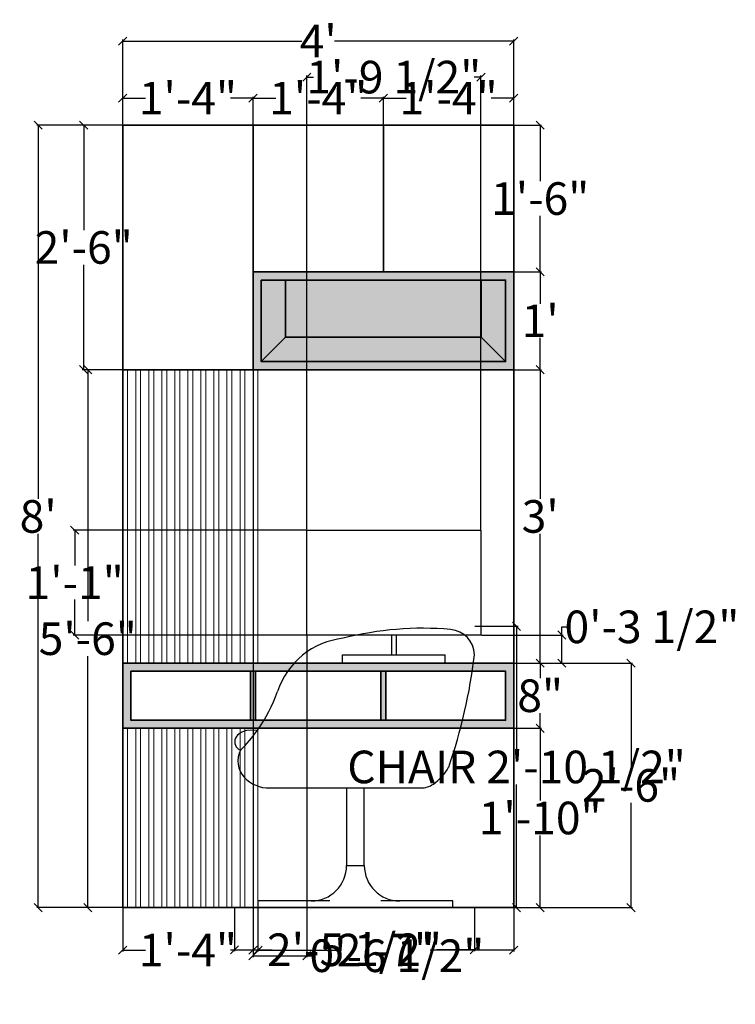
# Model space of a CAD drawing. Units: inches. Extents: x 1 to 89, y 9 to 130.
import ezdxf

# ---------------------------------------------------------------- set-up
doc = ezdxf.new("R2010")
doc.units = ezdxf.units.IN
doc.header["$MEASUREMENT"] = 0
for name, color, linetype, lineweight in [('A-ANNO-DIMS', 2, 'Continuous', 18), ('A-ELEV', 7, 'Continuous', 35), ('A-ELEV-PATT', 8, 'Continuous', 13), ('A-FURN', 8, 'Continuous', 25)]:
    doc.layers.add(name, color=color, linetype=linetype, lineweight=lineweight)
doc.styles.get("Standard").update_dxf_attribs({"font": 'arial.ttf'})
doc.dimstyles.get("Standard").update_dxf_attribs({"dimtxt": 4, "dimasz": 1, "dimexe": 0.18, "dimexo": 0.0625, "dimgap": 0.09, "dimtad": 0, "dimtih": 1, "dimtoh": 1, "dimdec": 0, "dimzin": 0, "dimdsep": 46, "dimlunit": 4, "dimtxsty": 'Standard', "dimblk": 'OBLIQUE', "dimcen": 0.09, "dimadec": 0, "dimazin": 0, "dimtfac": 1, "dimtdec": 0, "dimtofl": 0, "dimtmove": 0, "dimatfit": 3, "dimldrblk": 'OBLIQUE', "dimfxl": 1, "dimtolj": 1, "dimtzin": 0, "dimarcsym": 0})

# ---------------------------------------------------------------- blocks, each defined once
blk = doc.blocks.new('A$C2F5F5597')
at = {"ltscale": 20}
for p, q in [((51.1, 400), (27.4, 399.3)), ((79, 270), (252.2, 270)), ((252.2, 270), (252.2, 95)), ((292.2, 95), (292.2, 270)), ((292.2, 270), (419.9, 270)), ((252.2, 95), (292.2, 95)), ((172.2, 15), (52.2, 15)), ((52.2, 15), (52.2, 0)), ((214.7, 15), (52.2, 15)), ((52.2, 0), (492.2, 0)), ((492.2, 15), (329.7, 15)), ((492.2, 15), (372.2, 15)), ((492.2, 0), (492.2, 15))]:
    blk.add_line(p, q, dxfattribs=at)
blk.add_line((252.2, 270), (292.2, 270))
for centre, radius, start, end in [((424, -95.9), 726, 85.0159, 104.3072), ((482.6, 569.3), 58.2, 1.2474, 85.5637), ((264.6, 431.4), 177.3, 96.4526, 161.6024), ((-670.9, 714.7), 1220.3, 340.9618, 353.2158), ((-231.8, 601.9), 347.5, 324.4887, 340.7516), ((-231.8, 601.9), 347.5, 314.7292, 324.4887), ((20.7, 374.3), 20.9, 157.0939, 247.6023), ((31.5, 364.8), 34.8, 96.6901, 149.4967), ((60.1, 330.5), 53.3, 152.6544, 222.8556), ((385.8, 370), 110.5, 304.2659, 331.155), ((77, 346.6), 76.7, 223.0738, 271.4724), ((419.9, 320), 50, 270, 304.2659), ((172.2, 95), 80, 270, 0), ((372.2, 95), 80, 180, 270)]:
    blk.add_arc(centre, radius, start, end, dxfattribs=at)
blk = doc.blocks.new('_Oblique')
at = {"color": 0, "linetype": 'ByBlock', "lineweight": -2}
blk.add_line((-0.5, -0.5), (0.5, 0.5), dxfattribs=at)
blk = doc.blocks.new('*D3')
at = {"layer": 'A-ANNO-DIMS', "color": 0, "lineweight": -2, "transparency": 16777216}
for p, q in [((13.37, 116.69), (13.37, 127.12)), ((13.37, 126.94), (35.36, 126.94)), ((61.37, 126.94), (39.38, 126.94)), ((61.37, 116.69), (61.37, 127.12))]:
    blk.add_line(p, q, dxfattribs=at)
at = {"layer": 'Defpoints', "color": 0, "transparency": 16777216}
for p in [(61.37, 126.94), (13.37, 116.62), (61.37, 116.62)]:
    blk.add_point(p, dxfattribs=at)
at = {"layer": 'A-ANNO-DIMS', "color": 0, "lineweight": -2, "transparency": 16777216, "rotation": 180}
blk.add_blockref('_Oblique', (13.37, 126.94), dxfattribs=at)
at = {"layer": 'A-ANNO-DIMS', "color": 0, "lineweight": -2, "transparency": 16777216}
blk.add_blockref('_Oblique', (61.37, 126.94), dxfattribs=at)
at = {"layer": 'A-ANNO-DIMS', "color": 0, "transparency": 16777216, "insert": (37.37, 126.94), "char_height": 4, "attachment_point": 5}
blk.add_mtext("\\A1;4'", dxfattribs=at)
blk = doc.blocks.new('*D4')
at = {"layer": 'A-ANNO-DIMS', "color": 0, "lineweight": -2, "transparency": 16777216}
for p, q in [((13.37, 116.69), (13.37, 120.12)), ((13.37, 119.94), (16.15, 119.94)), ((29.37, 119.94), (26.59, 119.94)), ((29.37, 116.69), (29.37, 120.12))]:
    blk.add_line(p, q, dxfattribs=at)
at = {"layer": 'Defpoints', "color": 0, "transparency": 16777216}
for p in [(29.37, 119.94), (13.37, 116.62), (29.37, 116.62)]:
    blk.add_point(p, dxfattribs=at)
at = {"layer": 'A-ANNO-DIMS', "color": 0, "lineweight": -2, "transparency": 16777216, "rotation": 180}
blk.add_blockref('_Oblique', (13.37, 119.94), dxfattribs=at)
at = {"layer": 'A-ANNO-DIMS', "color": 0, "lineweight": -2, "transparency": 16777216}
blk.add_blockref('_Oblique', (29.37, 119.94), dxfattribs=at)
at = {"layer": 'A-ANNO-DIMS', "color": 0, "transparency": 16777216, "insert": (21.37, 119.94), "char_height": 4, "attachment_point": 5}
blk.add_mtext('\\A1;1\'-4"', dxfattribs=at)
blk = doc.blocks.new('*D5')
at = {"layer": 'A-ANNO-DIMS', "color": 0, "lineweight": -2, "transparency": 16777216}
for p, q in [((29.37, 116.69), (29.37, 120.12)), ((29.37, 119.94), (32.15, 119.94)), ((45.37, 119.94), (42.59, 119.94)), ((45.37, 116.69), (45.37, 120.12))]:
    blk.add_line(p, q, dxfattribs=at)
at = {"layer": 'Defpoints', "color": 0, "transparency": 16777216}
for p in [(45.37, 119.94), (29.37, 116.62), (45.37, 116.62)]:
    blk.add_point(p, dxfattribs=at)
at = {"layer": 'A-ANNO-DIMS', "color": 0, "lineweight": -2, "transparency": 16777216, "rotation": 180}
blk.add_blockref('_Oblique', (29.37, 119.94), dxfattribs=at)
at = {"layer": 'A-ANNO-DIMS', "color": 0, "lineweight": -2, "transparency": 16777216}
blk.add_blockref('_Oblique', (45.37, 119.94), dxfattribs=at)
at = {"layer": 'A-ANNO-DIMS', "color": 0, "transparency": 16777216, "insert": (37.37, 119.94), "char_height": 4, "attachment_point": 5}
blk.add_mtext('\\A1;1\'-4"', dxfattribs=at)
blk = doc.blocks.new('*D6')
at = {"layer": 'A-ANNO-DIMS', "color": 0, "lineweight": -2, "transparency": 16777216}
for p, q in [((45.37, 116.69), (45.37, 120.12)), ((45.37, 119.94), (48.15, 119.94)), ((61.37, 119.94), (58.59, 119.94)), ((61.37, 116.69), (61.37, 120.12))]:
    blk.add_line(p, q, dxfattribs=at)
at = {"layer": 'Defpoints', "color": 0, "transparency": 16777216}
for p in [(61.37, 119.94), (45.37, 116.62), (61.37, 116.62)]:
    blk.add_point(p, dxfattribs=at)
at = {"layer": 'A-ANNO-DIMS', "color": 0, "lineweight": -2, "transparency": 16777216, "rotation": 180}
blk.add_blockref('_Oblique', (45.37, 119.94), dxfattribs=at)
at = {"layer": 'A-ANNO-DIMS', "color": 0, "lineweight": -2, "transparency": 16777216}
blk.add_blockref('_Oblique', (61.37, 119.94), dxfattribs=at)
at = {"layer": 'A-ANNO-DIMS', "color": 0, "transparency": 16777216, "insert": (53.37, 119.94), "char_height": 4, "attachment_point": 5}
blk.add_mtext('\\A1;1\'-4"', dxfattribs=at)
blk = doc.blocks.new('*D7')
at = {"layer": 'A-ANNO-DIMS', "color": 0, "lineweight": -2, "transparency": 16777216}
for p, q in [((61.43, 116.62), (64.8, 116.62)), ((64.62, 116.62), (64.62, 109.76)), ((64.62, 98.62), (64.62, 105.49)), ((61.43, 98.62), (64.8, 98.62))]:
    blk.add_line(p, q, dxfattribs=at)
at = {"layer": 'Defpoints', "color": 0, "transparency": 16777216}
for p in [(61.37, 116.62), (61.37, 98.62), (64.62, 98.62)]:
    blk.add_point(p, dxfattribs=at)
at = {"layer": 'A-ANNO-DIMS', "color": 0, "lineweight": -2, "transparency": 16777216}
for p, rotation in [((64.62, 116.62), 90), ((64.62, 98.62), 270)]:
    blk.add_blockref('_Oblique', p, dxfattribs=dict(at, rotation=rotation))
at = {"layer": 'A-ANNO-DIMS', "color": 0, "transparency": 16777216, "insert": (64.62, 107.62), "char_height": 4, "attachment_point": 5}
blk.add_mtext('\\A1;1\'-6"', dxfattribs=at)
blk = doc.blocks.new('*D8')
at = {"layer": 'A-ANNO-DIMS', "color": 0, "lineweight": -2, "transparency": 16777216}
for p, q in [((61.43, 98.62), (64.8, 98.62)), ((64.62, 98.62), (64.62, 94.72)), ((64.62, 86.62), (64.62, 90.53)), ((61.43, 86.62), (64.8, 86.62))]:
    blk.add_line(p, q, dxfattribs=at)
at = {"layer": 'Defpoints', "color": 0, "transparency": 16777216}
for p in [(61.37, 98.62), (64.62, 98.62), (61.37, 86.62)]:
    blk.add_point(p, dxfattribs=at)
at = {"layer": 'A-ANNO-DIMS', "color": 0, "lineweight": -2, "transparency": 16777216}
for p, rotation in [((64.62, 98.62), 90), ((64.62, 86.62), 270)]:
    blk.add_blockref('_Oblique', p, dxfattribs=dict(at, rotation=rotation))
at = {"layer": 'A-ANNO-DIMS', "color": 0, "transparency": 16777216, "insert": (64.62, 92.62), "char_height": 4, "attachment_point": 5}
blk.add_mtext("\\A1;1'", dxfattribs=at)
blk = doc.blocks.new('*D9')
at = {"layer": 'A-ANNO-DIMS', "color": 0, "lineweight": -2, "transparency": 16777216}
for p, q in [((61.43, 86.62), (64.8, 86.62)), ((64.62, 86.62), (64.62, 70.76)), ((64.62, 50.62), (64.62, 66.49)), ((61.43, 50.62), (64.8, 50.62))]:
    blk.add_line(p, q, dxfattribs=at)
at = {"layer": 'Defpoints', "color": 0, "transparency": 16777216}
for p in [(61.37, 86.62), (61.37, 50.62), (64.62, 50.62)]:
    blk.add_point(p, dxfattribs=at)
at = {"layer": 'A-ANNO-DIMS', "color": 0, "lineweight": -2, "transparency": 16777216}
for p, rotation in [((64.62, 86.62), 90), ((64.62, 50.62), 270)]:
    blk.add_blockref('_Oblique', p, dxfattribs=dict(at, rotation=rotation))
at = {"layer": 'A-ANNO-DIMS', "color": 0, "transparency": 16777216, "insert": (64.62, 68.62), "char_height": 4, "attachment_point": 5}
blk.add_mtext("\\A1;3'", dxfattribs=at)
blk = doc.blocks.new('*D10')
at = {"layer": 'A-ANNO-DIMS', "color": 0, "lineweight": -2, "transparency": 16777216}
for p, q in [((61.43, 50.62), (64.8, 50.62)), ((64.62, 50.62), (64.62, 48.76)), ((64.62, 42.62), (64.62, 44.49)), ((61.43, 42.62), (64.8, 42.62))]:
    blk.add_line(p, q, dxfattribs=at)
at = {"layer": 'Defpoints', "color": 0, "transparency": 16777216}
for p in [(61.37, 50.62), (61.37, 42.62), (64.62, 42.62)]:
    blk.add_point(p, dxfattribs=at)
at = {"layer": 'A-ANNO-DIMS', "color": 0, "lineweight": -2, "transparency": 16777216}
for p, rotation in [((64.62, 50.62), 90), ((64.62, 42.62), 270)]:
    blk.add_blockref('_Oblique', p, dxfattribs=dict(at, rotation=rotation))
at = {"layer": 'A-ANNO-DIMS', "color": 0, "transparency": 16777216, "insert": (64.62, 46.62), "char_height": 4, "attachment_point": 5}
blk.add_mtext('\\A1;8"', dxfattribs=at)
blk = doc.blocks.new('*D11')
at = {"layer": 'A-ANNO-DIMS', "color": 0, "lineweight": -2, "transparency": 16777216}
for p, q in [((61.43, 42.62), (64.8, 42.62)), ((64.62, 42.62), (64.62, 33.76)), ((64.62, 20.62), (64.62, 29.49)), ((61.43, 20.62), (64.8, 20.62))]:
    blk.add_line(p, q, dxfattribs=at)
at = {"layer": 'Defpoints', "color": 0, "transparency": 16777216}
for p in [(61.37, 42.62), (61.37, 20.62), (64.62, 20.62)]:
    blk.add_point(p, dxfattribs=at)
at = {"layer": 'A-ANNO-DIMS', "color": 0, "lineweight": -2, "transparency": 16777216}
for p, rotation in [((64.62, 42.62), 90), ((64.62, 20.62), 270)]:
    blk.add_blockref('_Oblique', p, dxfattribs=dict(at, rotation=rotation))
at = {"layer": 'A-ANNO-DIMS', "color": 0, "transparency": 16777216, "insert": (64.62, 31.62), "char_height": 4, "attachment_point": 5}
blk.add_mtext('\\A1;1\'-10"', dxfattribs=at)
blk = doc.blocks.new('*D12')
at = {"layer": 'A-ANNO-DIMS', "color": 0, "lineweight": -2, "transparency": 16777216}
for p, q in [((61.43, 50.62), (75.95, 50.62)), ((75.77, 50.62), (75.77, 37.76)), ((75.77, 20.62), (75.77, 33.49)), ((61.43, 20.62), (75.95, 20.62))]:
    blk.add_line(p, q, dxfattribs=at)
at = {"layer": 'Defpoints', "color": 0, "transparency": 16777216}
for p in [(61.37, 50.62), (61.37, 20.62), (75.77, 20.62)]:
    blk.add_point(p, dxfattribs=at)
at = {"layer": 'A-ANNO-DIMS', "color": 0, "lineweight": -2, "transparency": 16777216}
for p, rotation in [((75.77, 50.62), 90), ((75.77, 20.62), 270)]:
    blk.add_blockref('_Oblique', p, dxfattribs=dict(at, rotation=rotation))
at = {"layer": 'A-ANNO-DIMS', "color": 0, "transparency": 16777216, "insert": (75.77, 35.62), "char_height": 4, "attachment_point": 5}
blk.add_mtext('\\A1;2\'-6"', dxfattribs=at)
blk = doc.blocks.new('*D13')
at = {"layer": 'A-ANNO-DIMS', "color": 0, "lineweight": -2, "transparency": 16777216}
for p, q in [((29.37, 86.56), (29.37, 15.23)), ((13.37, 20.56), (13.37, 15.23)), ((13.37, 15.41), (16.15, 15.41)), ((29.37, 15.41), (26.59, 15.41))]:
    blk.add_line(p, q, dxfattribs=at)
at = {"layer": 'Defpoints', "color": 0, "transparency": 16777216}
for p in [(29.37, 86.62), (13.37, 20.62), (29.37, 15.41)]:
    blk.add_point(p, dxfattribs=at)
at = {"layer": 'A-ANNO-DIMS', "color": 0, "lineweight": -2, "transparency": 16777216, "rotation": 180}
blk.add_blockref('_Oblique', (13.37, 15.41), dxfattribs=at)
at = {"layer": 'A-ANNO-DIMS', "color": 0, "lineweight": -2, "transparency": 16777216}
blk.add_blockref('_Oblique', (29.37, 15.41), dxfattribs=at)
at = {"layer": 'A-ANNO-DIMS', "color": 0, "transparency": 16777216, "insert": (21.37, 15.41), "char_height": 4, "attachment_point": 5}
blk.add_mtext('\\A1;1\'-4"', dxfattribs=at)
blk = doc.blocks.new('*D14')
at = {"layer": 'A-ANNO-DIMS', "color": 0, "lineweight": -2, "transparency": 16777216}
for p, q in [((61.37, 86.56), (61.37, 15.23)), ((29.97, 20.56), (29.97, 15.23)), ((29.97, 15.41), (40.23, 15.41)), ((61.37, 15.41), (51.11, 15.41))]:
    blk.add_line(p, q, dxfattribs=at)
at = {"layer": 'Defpoints', "color": 0, "transparency": 16777216}
for p in [(61.37, 86.62), (29.97, 20.62), (61.37, 15.41)]:
    blk.add_point(p, dxfattribs=at)
at = {"layer": 'A-ANNO-DIMS', "color": 0, "lineweight": -2, "transparency": 16777216, "rotation": 180}
blk.add_blockref('_Oblique', (29.97, 15.41), dxfattribs=at)
at = {"layer": 'A-ANNO-DIMS', "color": 0, "lineweight": -2, "transparency": 16777216}
blk.add_blockref('_Oblique', (61.37, 15.41), dxfattribs=at)
at = {"layer": 'A-ANNO-DIMS', "color": 0, "transparency": 16777216, "insert": (45.67, 15.41), "char_height": 4, "attachment_point": 5}
blk.add_mtext('\\A1;2\'-7"', dxfattribs=at)
blk = doc.blocks.new('*D15')
at = {"layer": 'A-ANNO-DIMS', "color": 0, "lineweight": -2, "transparency": 16777216}
for p, q in [((13.31, 86.62), (8.9, 86.62)), ((9.08, 86.62), (9.08, 55.76)), ((9.08, 20.62), (9.08, 51.49)), ((13.31, 20.62), (8.9, 20.62))]:
    blk.add_line(p, q, dxfattribs=at)
at = {"layer": 'Defpoints', "color": 0, "transparency": 16777216}
for p in [(13.37, 86.62), (9.08, 20.62), (13.37, 20.62)]:
    blk.add_point(p, dxfattribs=at)
at = {"layer": 'A-ANNO-DIMS', "color": 0, "lineweight": -2, "transparency": 16777216}
for p, rotation in [((9.08, 86.62), 90), ((9.08, 20.62), 270)]:
    blk.add_blockref('_Oblique', p, dxfattribs=dict(at, rotation=rotation))
at = {"layer": 'A-ANNO-DIMS', "color": 0, "transparency": 16777216, "insert": (9.08, 53.62), "char_height": 4, "attachment_point": 5}
blk.add_mtext('\\A1;5\'-6"', dxfattribs=at)
blk = doc.blocks.new('*D16')
at = {"layer": 'A-ANNO-DIMS', "color": 0, "lineweight": -2, "transparency": 16777216}
for p, q in [((13.31, 116.62), (8.4, 116.62)), ((8.58, 116.62), (8.58, 103.76)), ((8.58, 86.62), (8.58, 99.49)), ((13.31, 86.62), (8.4, 86.62))]:
    blk.add_line(p, q, dxfattribs=at)
at = {"layer": 'Defpoints', "color": 0, "transparency": 16777216}
for p in [(13.37, 116.62), (8.58, 86.62), (13.37, 86.62)]:
    blk.add_point(p, dxfattribs=at)
at = {"layer": 'A-ANNO-DIMS', "color": 0, "lineweight": -2, "transparency": 16777216}
for p, rotation in [((8.58, 116.62), 90), ((8.58, 86.62), 270)]:
    blk.add_blockref('_Oblique', p, dxfattribs=dict(at, rotation=rotation))
at = {"layer": 'A-ANNO-DIMS', "color": 0, "transparency": 16777216, "insert": (8.58, 101.62), "char_height": 4, "attachment_point": 5}
blk.add_mtext('\\A1;2\'-6"', dxfattribs=at)
blk = doc.blocks.new('*D17')
at = {"layer": 'A-ANNO-DIMS', "color": 0, "lineweight": -2, "transparency": 16777216}
for p, q in [((13.31, 116.62), (2.81, 116.62)), ((2.99, 116.62), (2.99, 70.76)), ((2.99, 20.62), (2.99, 66.49)), ((13.91, 20.62), (2.81, 20.62))]:
    blk.add_line(p, q, dxfattribs=at)
at = {"layer": 'Defpoints', "color": 0, "transparency": 16777216}
for p in [(13.37, 116.62), (2.99, 20.62), (13.97, 20.62)]:
    blk.add_point(p, dxfattribs=at)
at = {"layer": 'A-ANNO-DIMS', "color": 0, "lineweight": -2, "transparency": 16777216}
for p, rotation in [((2.99, 116.62), 90), ((2.99, 20.62), 270)]:
    blk.add_blockref('_Oblique', p, dxfattribs=dict(at, rotation=rotation))
at = {"layer": 'A-ANNO-DIMS', "color": 0, "transparency": 16777216, "insert": (2.99, 68.62), "char_height": 4, "attachment_point": 5}
blk.add_mtext("\\A1;8'", dxfattribs=at)
blk = doc.blocks.new('*D18')
at = {"layer": 'A-ANNO-DIMS', "color": 0, "lineweight": -2, "transparency": 16777216}
for p, q in [((56.61, 55.14), (61.9, 55.14)), ((61.72, 55.14), (61.72, 40.04)), ((61.72, 20.62), (61.72, 35.72)), ((56.61, 20.62), (61.9, 20.62))]:
    blk.add_line(p, q, dxfattribs=at)
at = {"layer": 'Defpoints', "color": 0, "transparency": 16777216}
for p in [(56.54, 55.14), (61.72, 55.14), (56.54, 20.62)]:
    blk.add_point(p, dxfattribs=at)
at = {"layer": 'A-ANNO-DIMS', "color": 0, "lineweight": -2, "transparency": 16777216}
for p, rotation in [((61.72, 55.14), 90), ((61.72, 20.62), 270)]:
    blk.add_blockref('_Oblique', p, dxfattribs=dict(at, rotation=rotation))
at = {"layer": 'A-ANNO-DIMS', "color": 0, "transparency": 16777216, "insert": (61.72, 37.88), "char_height": 4, "attachment_point": 5}
blk.add_mtext('\\A1;CHAIR 2\'-10 1/2"', dxfattribs=at)
blk = doc.blocks.new('*D19')
at = {"layer": 'A-ANNO-DIMS', "color": 0, "lineweight": -2, "transparency": 16777216}
for p, q in [((27.09, 20.56), (27.09, 15.27)), ((56.54, 20.56), (56.54, 15.27)), ((27.09, 15.45), (31.72, 15.45)), ((56.54, 15.45), (51.92, 15.45))]:
    blk.add_line(p, q, dxfattribs=at)
at = {"layer": 'Defpoints', "color": 0, "transparency": 16777216}
for p in [(27.09, 20.62), (56.54, 20.62), (56.54, 15.45)]:
    blk.add_point(p, dxfattribs=at)
at = {"layer": 'A-ANNO-DIMS', "color": 0, "lineweight": -2, "transparency": 16777216, "rotation": 180}
blk.add_blockref('_Oblique', (27.09, 15.45), dxfattribs=at)
at = {"layer": 'A-ANNO-DIMS', "color": 0, "lineweight": -2, "transparency": 16777216}
blk.add_blockref('_Oblique', (56.54, 15.45), dxfattribs=at)
at = {"layer": 'A-ANNO-DIMS', "color": 0, "transparency": 16777216, "insert": (41.82, 15.45), "char_height": 4, "attachment_point": 5}
blk.add_mtext('\\A1;2\'-5 1/2"', dxfattribs=at)
blk = doc.blocks.new('*D20')
at = {"layer": 'A-ANNO-DIMS', "color": 0, "lineweight": -2, "transparency": 16777216}
for p, q in [((35.96, 67), (35.96, 122.7)), ((35.96, 122.52), (36.78, 122.52)), ((57.35, 122.52), (56.53, 122.52)), ((57.35, 67), (57.35, 122.7))]:
    blk.add_line(p, q, dxfattribs=at)
at = {"layer": 'Defpoints', "color": 0, "transparency": 16777216}
for p in [(57.35, 122.52), (35.96, 66.93), (57.35, 66.93)]:
    blk.add_point(p, dxfattribs=at)
at = {"layer": 'A-ANNO-DIMS', "color": 0, "lineweight": -2, "transparency": 16777216, "rotation": 180}
blk.add_blockref('_Oblique', (35.96, 122.52), dxfattribs=at)
at = {"layer": 'A-ANNO-DIMS', "color": 0, "lineweight": -2, "transparency": 16777216}
blk.add_blockref('_Oblique', (57.35, 122.52), dxfattribs=at)
at = {"layer": 'A-ANNO-DIMS', "color": 0, "transparency": 16777216, "insert": (46.65, 122.52), "char_height": 4, "attachment_point": 5}
blk.add_mtext('\\A1;1\'-9 1/2"', dxfattribs=at)
blk = doc.blocks.new('*D21')
at = {"layer": 'A-ANNO-DIMS', "color": 0, "lineweight": -2, "transparency": 16777216}
for p, q in [((35.9, 66.93), (7.29, 66.93)), ((7.47, 66.93), (7.47, 62.6)), ((7.47, 54.07), (7.47, 58.41)), ((35.9, 54.07), (7.29, 54.07))]:
    blk.add_line(p, q, dxfattribs=at)
at = {"layer": 'Defpoints', "color": 0, "transparency": 16777216}
for p in [(7.47, 66.93), (35.96, 66.93), (35.96, 54.07)]:
    blk.add_point(p, dxfattribs=at)
at = {"layer": 'A-ANNO-DIMS', "color": 0, "lineweight": -2, "transparency": 16777216}
for p, rotation in [((7.47, 66.93), 90), ((7.47, 54.07), 270)]:
    blk.add_blockref('_Oblique', p, dxfattribs=dict(at, rotation=rotation))
at = {"layer": 'A-ANNO-DIMS', "color": 0, "transparency": 16777216, "insert": (7.47, 60.5), "char_height": 4, "attachment_point": 5}
blk.add_mtext('\\A1;1\'-1"', dxfattribs=at)
blk = doc.blocks.new('*D22')
at = {"layer": 'A-ANNO-DIMS', "color": 0, "lineweight": -2, "transparency": 16777216}
for p, q in [((67.27, 54.07), (67.27, 55.07)), ((67.27, 55.07), (68.27, 55.07)), ((57.41, 54.07), (67.45, 54.07)), ((67.27, 50.62), (67.27, 54.07)), ((61.43, 50.62), (67.45, 50.62))]:
    blk.add_line(p, q, dxfattribs=at)
at = {"layer": 'Defpoints', "color": 0, "transparency": 16777216}
for p in [(57.35, 54.07), (67.27, 54.07), (61.37, 50.62)]:
    blk.add_point(p, dxfattribs=at)
at = {"layer": 'A-ANNO-DIMS', "color": 0, "lineweight": -2, "transparency": 16777216}
for p, rotation in [((67.27, 54.07), 90), ((67.27, 50.62), 270)]:
    blk.add_blockref('_Oblique', p, dxfattribs=dict(at, rotation=rotation))
at = {"layer": 'A-ANNO-DIMS', "color": 0, "transparency": 16777216, "insert": (78.34, 55.07), "char_height": 4, "attachment_point": 5}
blk.add_mtext('\\A1;0\'-3 1/2"', dxfattribs=at)
blk = doc.blocks.new('*D23')
at = {"layer": 'A-ANNO-DIMS', "color": 0, "lineweight": -2, "transparency": 16777216}
for p, q in [((35.96, 54.01), (35.96, 14.54)), ((29.37, 50.56), (29.37, 14.54)), ((29.37, 14.72), (35.96, 14.72)), ((35.96, 14.72), (36.96, 14.72))]:
    blk.add_line(p, q, dxfattribs=at)
at = {"layer": 'Defpoints', "color": 0, "transparency": 16777216}
for p in [(35.96, 54.07), (29.37, 50.62), (35.96, 14.72)]:
    blk.add_point(p, dxfattribs=at)
at = {"layer": 'A-ANNO-DIMS', "color": 0, "lineweight": -2, "transparency": 16777216, "rotation": 180}
blk.add_blockref('_Oblique', (29.37, 14.72), dxfattribs=at)
at = {"layer": 'A-ANNO-DIMS', "color": 0, "lineweight": -2, "transparency": 16777216}
blk.add_blockref('_Oblique', (35.96, 14.72), dxfattribs=at)
at = {"layer": 'A-ANNO-DIMS', "color": 0, "transparency": 16777216, "insert": (47.03, 14.72), "char_height": 4, "attachment_point": 5}
blk.add_mtext('\\A1;0\'-6 1/2"', dxfattribs=at)

msp = doc.modelspace()

# ---------------------------------------------------------------- hatches: boundary and pattern name
at = {"layer": 'A-ELEV-PATT'}
h = msp.add_hatch(color=256, dxfattribs=at)
h.dxf.hatch_style = 1
h.paths.add_polyline_path([(13.37, 50.62), (13.37, 42.62), (61.37, 42.62), (61.37, 50.62)])
h.paths.add_polyline_path([(60.37, 49.62), (60.37, 43.62), (14.37, 43.62), (14.37, 49.62)], flags=16)
h.paths.add_polyline_path([(61.37, 86.62), (61.37, 98.62), (29.37, 98.62), (29.37, 86.62)])
h.paths.add_polyline_path([(30.37, 87.62), (30.37, 97.62), (60.37, 97.62), (60.37, 87.62)], flags=16)
h = msp.add_hatch(color=256, dxfattribs=at)
h.dxf.hatch_style = 1
h.paths.add_polyline_path([(61.37, 86.62), (61.37, 98.62), (29.37, 98.62), (29.37, 86.62)])
h.paths.add_polyline_path([(30.37, 87.62), (30.37, 97.62), (60.37, 97.62), (60.37, 87.62)], flags=16)
h.paths.add_polyline_path([(13.37, 50.62), (13.37, 42.62), (61.37, 42.62), (61.37, 50.62)])
h.paths.add_polyline_path([(60.37, 49.62), (60.37, 43.62), (14.37, 43.62), (14.37, 49.62)], flags=16)
h = msp.add_hatch(color=256, dxfattribs=at)
h.dxf.hatch_style = 1
h.paths.add_polyline_path([(33.37, 97.62), (30.37, 97.62), (30.37, 87.62), (33.37, 90.62)])
h.paths.add_polyline_path([(57.37, 90.62), (33.37, 90.62), (30.37, 87.62), (60.37, 87.62)])
h.paths.add_polyline_path([(60.37, 97.62), (57.37, 97.62), (57.37, 90.62), (60.37, 87.62)])
h = msp.add_hatch(color=256, dxfattribs=at)
h.dxf.hatch_style = 1
h.paths.add_polyline_path([(57.37, 90.62), (57.37, 97.62), (33.37, 97.62), (33.37, 90.62)])
h = msp.add_hatch(color=256, dxfattribs=at)
h.dxf.hatch_style = 1
h.paths.add_polyline_path([(29.07, 43.62), (29.67, 43.62), (29.67, 49.62), (29.07, 49.62)])
h.paths.add_polyline_path([(45.67, 49.62), (45.07, 49.62), (45.07, 43.62), (45.67, 43.62)])

# ---------------------------------------------------------------- linework, layer by layer
at = {"layer": 'A-ELEV'}
for p, q in [((13.37, 116.62), (61.37, 116.62)), ((13.37, 86.62), (13.37, 116.62)), ((29.37, 98.62), (29.37, 116.62)), ((45.37, 98.62), (45.37, 116.62)), ((61.37, 116.62), (61.37, 98.62)), ((61.37, 98.62), (61.37, 86.62)), ((30.37, 87.62), (33.37, 90.62)), ((60.37, 87.62), (57.37, 90.62)), ((13.37, 86.62), (61.37, 86.62)), ((13.37, 86.62), (13.37, 50.62)), ((61.37, 86.62), (61.37, 50.62)), ((13.37, 42.62), (13.37, 50.62)), ((13.37, 50.62), (13.37, 42.62)), ((29.07, 49.62), (29.07, 43.62)), ((29.67, 49.62), (29.67, 43.62)), ((45.07, 49.62), (45.07, 43.62)), ((45.67, 49.62), (45.67, 43.62)), ((61.37, 50.62), (61.37, 20.62))]:
    msp.add_line(p, q, dxfattribs=at)
for points in [[(29.37, 98.62), (29.37, 86.62), (61.37, 86.62), (61.37, 98.62)], [(30.37, 97.62), (30.37, 87.62), (60.37, 87.62), (60.37, 97.62)], [(13.37, 50.62), (61.37, 50.62), (61.37, 42.62), (13.37, 42.62)], [(14.37, 49.62), (60.37, 49.62), (60.37, 43.62), (14.37, 43.62)]]:
    msp.add_lwpolyline(points, close=True, dxfattribs=at)
for points in [[(33.37, 97.62), (33.37, 90.62), (57.37, 90.62), (57.37, 97.62)], [(13.37, 42.62), (13.37, 20.62), (61.37, 20.62)]]:
    msp.add_lwpolyline(points, dxfattribs=at)
at = {"layer": 'A-ELEV-PATT'}
for p, q in [((13.97, 86.62), (13.97, 50.62)), ((14.97, 86.62), (14.97, 50.62)), ((15.57, 86.62), (15.57, 50.62)), ((16.57, 86.62), (16.57, 50.62)), ((17.17, 86.62), (17.17, 50.62)), ((18.17, 86.62), (18.17, 50.62)), ((18.77, 86.62), (18.77, 50.62)), ((19.77, 86.62), (19.77, 50.62)), ((20.37, 86.62), (20.37, 50.62)), ((21.37, 86.62), (21.37, 50.62)), ((21.97, 86.62), (21.97, 50.62)), ((22.97, 86.62), (22.97, 50.62)), ((23.57, 86.62), (23.57, 50.62)), ((24.57, 86.62), (24.57, 50.62)), ((25.17, 86.62), (25.17, 50.62)), ((26.17, 86.62), (26.17, 50.62)), ((26.77, 86.62), (26.77, 50.62)), ((27.77, 86.62), (27.77, 50.62)), ((28.37, 86.62), (28.37, 50.62)), ((29.37, 86.62), (29.37, 50.62)), ((29.97, 86.62), (29.97, 50.62)), ((13.97, 42.62), (13.97, 20.62)), ((14.97, 42.62), (14.97, 20.62)), ((15.57, 42.62), (15.57, 20.62)), ((16.57, 42.62), (16.57, 20.62)), ((17.17, 42.62), (17.17, 20.62)), ((18.17, 42.62), (18.17, 20.62)), ((18.77, 42.62), (18.77, 20.62)), ((19.77, 42.62), (19.77, 20.62)), ((20.37, 42.62), (20.37, 20.62)), ((21.37, 42.62), (21.37, 20.62)), ((21.97, 42.62), (21.97, 20.62)), ((22.97, 42.62), (22.97, 20.62)), ((23.57, 42.62), (23.57, 20.62)), ((24.57, 42.62), (24.57, 20.62)), ((25.17, 42.62), (25.17, 20.62)), ((26.17, 42.62), (26.17, 20.62)), ((26.77, 42.62), (26.77, 20.62)), ((27.77, 42.62), (27.77, 20.62)), ((28.37, 42.62), (28.37, 20.62)), ((29.37, 42.62), (29.37, 20.62)), ((29.97, 42.62), (29.97, 20.62))]:
    msp.add_line(p, q, dxfattribs=at)
at = {"layer": 'A-FURN'}
for p, q in [((46.35, 54.07), (46.35, 51.62)), ((46.95, 54.07), (46.95, 51.62)), ((40.35, 50.62), (40.35, 51.62)), ((40.35, 51.62), (52.95, 51.62)), ((52.95, 50.62), (52.95, 51.62)), ((46.35, 50.62), (40.35, 50.62)), ((46.95, 50.62), (52.95, 50.62))]:
    msp.add_line(p, q, dxfattribs=at)
msp.add_lwpolyline([(35.96, 66.93), (57.35, 66.93), (57.35, 54.07), (35.96, 54.07)], close=True, dxfattribs=at)

# ---------------------------------------------------------------- block references
at = {"layer": 'A-FURN', "xscale": 0.0543986261010282, "yscale": 0.0543986261010282, "zscale": 0.0543986261010282}
msp.add_blockref('A$C2F5F5597', (27.13, 20.62), dxfattribs=at)

# ---------------------------------------------------------------- dimensions: what is measured, and where the dimension line sits
at = {"layer": 'A-ANNO-DIMS'}
for base, p1, p2, override, picture, middle in [((61.37, 126.94), (13.37, 116.62), (61.37, 116.62), {"dimclrd": 0, "dimclre": 0, "dimclrt": 0}, '*D3', (37.37, 126.94)), ((57.35, 122.52), (35.96, 66.93), (57.35, 66.93), {"dimdec": 1, "dimlfac": 1, "dimrnd": 0, "dimzin": 1, "dimdsep": 46, "dimlunit": 4, "dimfrac": 2}, '*D20', (46.65, 122.52)), ((29.37, 119.94), (13.37, 116.62), (29.37, 116.62), {"dimclrd": 0, "dimclre": 0, "dimclrt": 0}, '*D4', (21.37, 119.94)), ((45.37, 119.94), (29.37, 116.62), (45.37, 116.62), {"dimclrd": 0, "dimclre": 0, "dimclrt": 0}, '*D5', (37.37, 119.94)), ((61.37, 119.94), (45.37, 116.62), (61.37, 116.62), {"dimclrd": 0, "dimclre": 0, "dimclrt": 0}, '*D6', (53.37, 119.94)), ((29.37, 15.41), (13.37, 20.62), (29.37, 86.62), {"dimclrd": 0, "dimclre": 0, "dimclrt": 0}, '*D13', (21.37, 15.41)), ((61.37, 15.41), (29.97, 20.62), (61.37, 86.62), {"dimclrd": 0, "dimclre": 0, "dimclrt": 0}, '*D14', (45.67, 15.41)), ((35.96, 14.72), (29.37, 50.62), (35.96, 54.07), {"dimdec": 1, "dimlfac": 1, "dimrnd": 0, "dimzin": 1, "dimdsep": 46, "dimlunit": 4, "dimfrac": 2}, '*D23', (47.03, 14.72)), ((56.545, 15.4466), (27.0873, 20.6236), (56.545, 20.6236), {"dimdec": 1, "dimrnd": 0, "dimzin": 1, "dimlunit": 4, "dimfrac": 2}, '*D19', (41.8162, 15.4466))]:
    dim = msp.add_linear_dim(base=base, p1=p1, p2=p2, dimstyle='Standard', override=override, dxfattribs=at)
    dim.commit()
    dim.dimension.update_dxf_attribs({"geometry": picture, "text_midpoint": middle})
for base, p1, p2, override, picture, middle in [((2.99, 20.62), (13.37, 116.62), (13.97, 20.62), {"dimclrd": 0, "dimclre": 0, "dimclrt": 0}, '*D17', (2.99, 68.62)), ((8.58, 86.62), (13.37, 116.62), (13.37, 86.62), {"dimclrd": 0, "dimclre": 0, "dimclrt": 0}, '*D16', (8.58, 101.62)), ((64.62, 98.62), (61.37, 116.62), (61.37, 98.62), {"dimclrd": 0, "dimclre": 0, "dimclrt": 0}, '*D7', (64.62, 107.62)), ((64.62, 98.62), (61.37, 86.62), (61.37, 98.62), {"dimclrd": 0, "dimclre": 0, "dimclrt": 0}, '*D8', (64.62, 92.62)), ((9.08, 20.62), (13.37, 86.62), (13.37, 20.62), {"dimclrd": 0, "dimclre": 0, "dimclrt": 0}, '*D15', (9.08, 53.62)), ((64.62, 50.62), (61.37, 86.62), (61.37, 50.62), {"dimclrd": 0, "dimclre": 0, "dimclrt": 0}, '*D9', (64.62, 68.62)), ((7.47, 66.93), (35.96, 54.07), (35.96, 66.93), {"dimdec": 1, "dimlfac": 1, "dimrnd": 0, "dimzin": 1, "dimdsep": 46, "dimlunit": 4, "dimfrac": 2}, '*D21', (7.47, 60.5)), ((67.2685, 54.072), (61.3685, 50.6236), (57.3455, 54.072), {"dimdec": 1, "dimlfac": 1, "dimrnd": 0, "dimzin": 1, "dimdsep": 46, "dimlunit": 4, "dimfrac": 2}, '*D22', (78.3353, 55.072)), ((64.62, 42.62), (61.37, 50.62), (61.37, 42.62), {"dimclrd": 0, "dimclre": 0, "dimclrt": 0}, '*D10', (64.62, 46.62)), ((75.77, 20.62), (61.37, 50.62), (61.37, 20.62), {"dimclrd": 0, "dimclre": 0, "dimclrt": 0}, '*D12', (75.77, 35.62)), ((64.62, 20.62), (61.37, 42.62), (61.37, 20.62), {"dimclrd": 0, "dimclre": 0, "dimclrt": 0}, '*D11', (64.62, 31.62))]:
    dim = msp.add_linear_dim(base=base, p1=p1, p2=p2, angle=90, dimstyle='Standard', override=override, dxfattribs=at)
    dim.commit()
    dim.dimension.update_dxf_attribs({"geometry": picture, "text_midpoint": middle})
dim = msp.add_linear_dim(base=(61.72, 55.14), p1=(56.54, 20.62), p2=(56.54, 55.14), angle=90, text='CHAIR <>', dimstyle='Standard', override={"dimdec": 1, "dimrnd": 0, "dimzin": 1, "dimlunit": 4, "dimfrac": 2}, dxfattribs=at)
dim.commit()
dim.dimension.update_dxf_attribs({"geometry": '*D18', "text_midpoint": (61.72, 37.88)})

doc.saveas('drawing.dxf')
